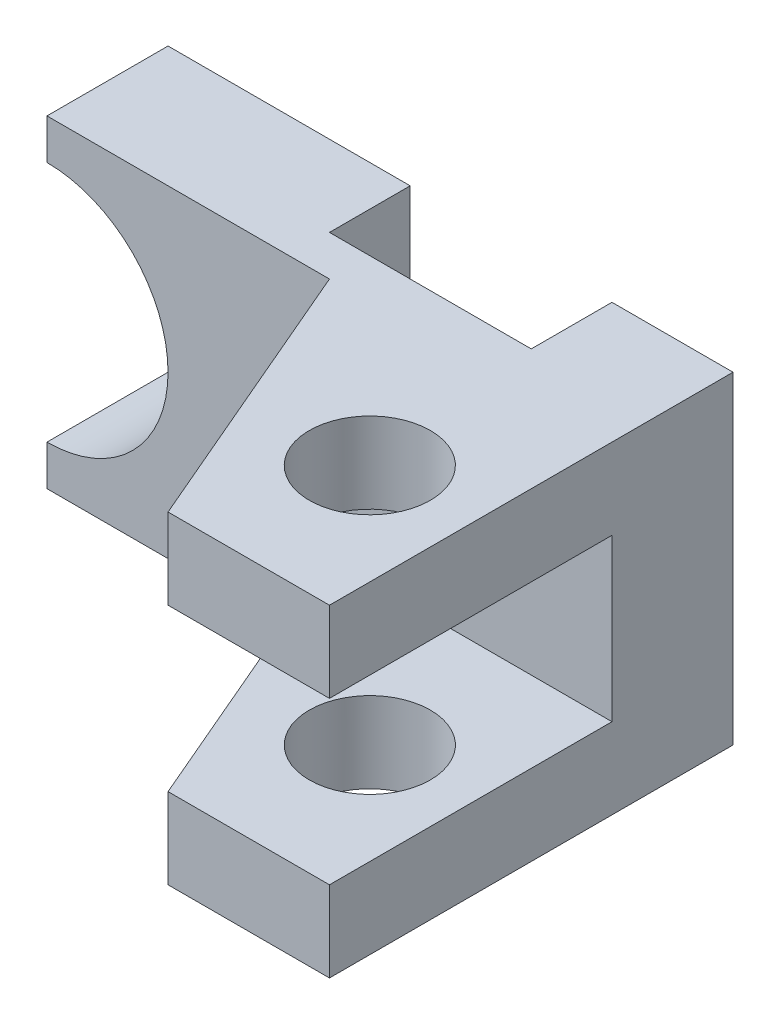
ISO-10303-21;
HEADER;
FILE_DESCRIPTION(('STEP AP214'),'2;1');
FILE_NAME('part.step','',(''),(''),'','','');
FILE_SCHEMA(('AUTOMOTIVE_DESIGN { 1 0 10303 214 1 1 1 1 }'));
ENDSEC;
DATA;
#1=APPLICATION_CONTEXT('core data for automotive mechanical design processes');
#2=APPLICATION_PROTOCOL_DEFINITION('international standard','automotive_design',2000,#1);
#3=PRODUCT_CONTEXT('',#1,'mechanical');
#4=PRODUCT('Part','Part','',(#3));
#5=PRODUCT_RELATED_PRODUCT_CATEGORY('part','',(#4));
#6=PRODUCT_DEFINITION_FORMATION('','',#4);
#7=PRODUCT_DEFINITION_CONTEXT('part definition',#1,'design');
#8=PRODUCT_DEFINITION('design','',#6,#7);
#9=PRODUCT_DEFINITION_SHAPE('','',#8);
#10=(LENGTH_UNIT() NAMED_UNIT(*) SI_UNIT(.MILLI.,.METRE.));
#11=(NAMED_UNIT(*) PLANE_ANGLE_UNIT() SI_UNIT($,.RADIAN.));
#12=(NAMED_UNIT(*) SI_UNIT($,.STERADIAN.) SOLID_ANGLE_UNIT());
#13=UNCERTAINTY_MEASURE_WITH_UNIT(LENGTH_MEASURE(1.E-05),#10,'distance_accuracy_value','');
#14=(GEOMETRIC_REPRESENTATION_CONTEXT(3) GLOBAL_UNCERTAINTY_ASSIGNED_CONTEXT((#13)) GLOBAL_UNIT_ASSIGNED_CONTEXT((#10,
#11,#12)) REPRESENTATION_CONTEXT('',''));
#15=CARTESIAN_POINT('',(0.,0.,0.));
#16=DIRECTION('',(0.,0.,1.));
#17=DIRECTION('',(1.,0.,0.));
#18=AXIS2_PLACEMENT_3D('',#15,#16,#17);
#19=CARTESIAN_POINT('',(0.,0.,0.));
#20=DIRECTION('',(0.,0.,1.));
#21=DIRECTION('',(1.,0.,0.));
#22=AXIS2_PLACEMENT_3D('',#19,#20,#21);
#23=PLANE('',#22);
#24=DIRECTION('',(-1.,0.,0.));
#25=VECTOR('',#24,1.);
#26=CARTESIAN_POINT('',(0.,0.,0.));
#27=LINE('',#26,#25);
#28=CARTESIAN_POINT('',(60.,0.,0.));
#29=VERTEX_POINT('',#28);
#30=CARTESIAN_POINT('',(0.,0.,0.));
#31=VERTEX_POINT('',#30);
#32=EDGE_CURVE('E279',#29,#31,#27,.T.);
#33=ORIENTED_EDGE('',*,*,#32,.F.);
#34=DIRECTION('',(0.,-1.,0.));
#35=VECTOR('',#34,1.);
#36=CARTESIAN_POINT('',(60.,0.,0.));
#37=LINE('',#36,#35);
#38=CARTESIAN_POINT('',(60.,-80.,0.));
#39=VERTEX_POINT('',#38);
#40=EDGE_CURVE('E192',#29,#39,#37,.T.);
#41=ORIENTED_EDGE('',*,*,#40,.T.);
#42=DIRECTION('',(1.,0.,0.));
#43=VECTOR('',#42,1.);
#44=CARTESIAN_POINT('',(0.,-80.,0.));
#45=LINE('',#44,#43);
#46=CARTESIAN_POINT('',(0.,-80.,0.));
#47=VERTEX_POINT('',#46);
#48=EDGE_CURVE('E272',#47,#39,#45,.T.);
#49=ORIENTED_EDGE('',*,*,#48,.F.);
#50=DIRECTION('',(0.,-1.,0.));
#51=VECTOR('',#50,1.);
#52=CARTESIAN_POINT('',(0.,0.,0.));
#53=LINE('',#52,#51);
#54=CARTESIAN_POINT('',(0.,-70.,0.));
#55=VERTEX_POINT('',#54);
#56=EDGE_CURVE('E269',#55,#47,#53,.T.);
#57=ORIENTED_EDGE('',*,*,#56,.F.);
#58=CARTESIAN_POINT('',(0.,-40.,0.));
#59=DIRECTION('',(0.,0.,1.));
#60=DIRECTION('',(1.,0.,0.));
#61=AXIS2_PLACEMENT_3D('',#58,#59,#60);
#62=CIRCLE('',#61,30.);
#63=CARTESIAN_POINT('',(0.,-10.,0.));
#64=VERTEX_POINT('',#63);
#65=EDGE_CURVE('E246',#55,#64,#62,.T.);
#66=ORIENTED_EDGE('',*,*,#65,.T.);
#67=EDGE_CURVE('E256',#31,#64,#53,.T.);
#68=ORIENTED_EDGE('',*,*,#67,.F.);
#69=EDGE_LOOP('',(#33,#41,#49,#57,#66,#68));
#70=FACE_BOUND('',#69,.T.);
#71=ADVANCED_FACE('F50',(#70),#23,.F.);
#72=CARTESIAN_POINT('',(0.,-40.,30.));
#73=DIRECTION('',(0.,0.,-1.));
#74=DIRECTION('',(-1.,0.,0.));
#75=AXIS2_PLACEMENT_3D('',#72,#73,#74);
#76=CYLINDRICAL_SURFACE('',#75,30.);
#77=ORIENTED_EDGE('',*,*,#65,.F.);
#78=DIRECTION('',(0.,0.,-1.));
#79=VECTOR('',#78,1.);
#80=CARTESIAN_POINT('',(0.,-70.,30.));
#81=LINE('',#80,#79);
#82=CARTESIAN_POINT('',(0.,-70.,30.));
#83=VERTEX_POINT('',#82);
#84=EDGE_CURVE('E11',#83,#55,#81,.T.);
#85=ORIENTED_EDGE('',*,*,#84,.F.);
#86=CARTESIAN_POINT('',(0.,-40.,30.));
#87=DIRECTION('',(0.,0.,1.));
#88=DIRECTION('',(1.,0.,0.));
#89=AXIS2_PLACEMENT_3D('',#86,#87,#88);
#90=CIRCLE('',#89,30.);
#91=CARTESIAN_POINT('',(0.,-10.,30.));
#92=VERTEX_POINT('',#91);
#93=EDGE_CURVE('E255',#83,#92,#90,.T.);
#94=ORIENTED_EDGE('',*,*,#93,.T.);
#95=DIRECTION('',(0.,0.,-1.));
#96=VECTOR('',#95,1.);
#97=CARTESIAN_POINT('',(0.,-10.,30.));
#98=LINE('',#97,#96);
#99=EDGE_CURVE('E278',#92,#64,#98,.T.);
#100=ORIENTED_EDGE('',*,*,#99,.T.);
#101=EDGE_LOOP('',(#77,#85,#94,#100));
#102=FACE_BOUND('',#101,.T.);
#103=ADVANCED_FACE('F47',(#102),#76,.F.);
#104=CARTESIAN_POINT('',(0.,0.,30.));
#105=DIRECTION('',(1.,0.,0.));
#106=DIRECTION('',(0.,0.,-1.));
#107=AXIS2_PLACEMENT_3D('',#104,#105,#106);
#108=PLANE('',#107);
#109=ORIENTED_EDGE('',*,*,#56,.T.);
#110=DIRECTION('',(0.,0.,-1.));
#111=VECTOR('',#110,1.);
#112=CARTESIAN_POINT('',(0.,-80.,30.));
#113=LINE('',#112,#111);
#114=CARTESIAN_POINT('',(0.,-80.,30.));
#115=VERTEX_POINT('',#114);
#116=EDGE_CURVE('E57',#115,#47,#113,.T.);
#117=ORIENTED_EDGE('',*,*,#116,.F.);
#118=DIRECTION('',(0.,-1.,0.));
#119=VECTOR('',#118,1.);
#120=CARTESIAN_POINT('',(0.,0.,30.));
#121=LINE('',#120,#119);
#122=EDGE_CURVE('E260',#83,#115,#121,.T.);
#123=ORIENTED_EDGE('',*,*,#122,.F.);
#124=ORIENTED_EDGE('',*,*,#84,.T.);
#125=EDGE_LOOP('',(#109,#117,#123,#124));
#126=FACE_BOUND('',#125,.T.);
#127=ADVANCED_FACE('F361',(#126),#108,.F.);
#128=CARTESIAN_POINT('',(0.,-80.,30.));
#129=DIRECTION('',(0.,1.,0.));
#130=DIRECTION('',(0.,0.,1.));
#131=AXIS2_PLACEMENT_3D('',#128,#129,#130);
#132=PLANE('',#131);
#133=CARTESIAN_POINT('',(115.,-80.,65.));
#134=DIRECTION('',(0.,-1.,0.));
#135=DIRECTION('',(0.,0.,-1.));
#136=AXIS2_PLACEMENT_3D('',#133,#134,#135);
#137=CIRCLE('',#136,15.);
#138=CARTESIAN_POINT('',(115.,-80.,50.));
#139=VERTEX_POINT('',#138);
#140=EDGE_CURVE('E191',#139,#139,#137,.T.);
#141=ORIENTED_EDGE('',*,*,#140,.F.);
#142=EDGE_LOOP('',(#141));
#143=FACE_BOUND('',#142,.T.);
#144=ORIENTED_EDGE('',*,*,#48,.T.);
#145=DIRECTION('',(0.,0.,-1.));
#146=VECTOR('',#145,1.);
#147=CARTESIAN_POINT('',(60.,-80.,20.));
#148=LINE('',#147,#146);
#149=CARTESIAN_POINT('',(60.,-80.,20.));
#150=VERTEX_POINT('',#149);
#151=EDGE_CURVE('E181',#150,#39,#148,.T.);
#152=ORIENTED_EDGE('',*,*,#151,.F.);
#153=DIRECTION('',(-1.,0.,0.));
#154=VECTOR('',#153,1.);
#155=CARTESIAN_POINT('',(110.,-80.,20.));
#156=LINE('',#155,#154);
#157=CARTESIAN_POINT('',(110.,-80.,20.));
#158=VERTEX_POINT('',#157);
#159=EDGE_CURVE('E183',#158,#150,#156,.T.);
#160=ORIENTED_EDGE('',*,*,#159,.F.);
#161=DIRECTION('',(0.,0.,1.));
#162=VECTOR('',#161,1.);
#163=CARTESIAN_POINT('',(110.,-80.,0.));
#164=LINE('',#163,#162);
#165=CARTESIAN_POINT('',(110.,-80.,0.));
#166=VERTEX_POINT('',#165);
#167=EDGE_CURVE('E162',#166,#158,#164,.T.);
#168=ORIENTED_EDGE('',*,*,#167,.F.);
#169=CARTESIAN_POINT('',(140.,-80.,0.));
#170=VERTEX_POINT('',#169);
#171=EDGE_CURVE('E275',#166,#170,#45,.T.);
#172=ORIENTED_EDGE('',*,*,#171,.T.);
#173=DIRECTION('',(0.,0.,-1.));
#174=VECTOR('',#173,1.);
#175=CARTESIAN_POINT('',(140.,-80.,30.));
#176=LINE('',#175,#174);
#177=CARTESIAN_POINT('',(140.,-80.,100.));
#178=VERTEX_POINT('',#177);
#179=EDGE_CURVE('E289',#178,#170,#176,.T.);
#180=ORIENTED_EDGE('',*,*,#179,.F.);
#181=DIRECTION('',(-1.,0.,0.));
#182=VECTOR('',#181,1.);
#183=CARTESIAN_POINT('',(140.,-80.,100.));
#184=LINE('',#183,#182);
#185=CARTESIAN_POINT('',(100.,-80.,100.));
#186=VERTEX_POINT('',#185);
#187=EDGE_CURVE('E223',#178,#186,#184,.T.);
#188=ORIENTED_EDGE('',*,*,#187,.T.);
#189=DIRECTION('',(-0.393919298579168,0.,-0.919145030018058));
#190=VECTOR('',#189,1.);
#191=CARTESIAN_POINT('',(70.,-80.,30.));
#192=LINE('',#191,#190);
#193=CARTESIAN_POINT('',(70.,-80.,30.));
#194=VERTEX_POINT('',#193);
#195=EDGE_CURVE('E235',#186,#194,#192,.T.);
#196=ORIENTED_EDGE('',*,*,#195,.T.);
#197=DIRECTION('',(1.,0.,0.));
#198=VECTOR('',#197,1.);
#199=CARTESIAN_POINT('',(0.,-80.,30.));
#200=LINE('',#199,#198);
#201=EDGE_CURVE('E257',#115,#194,#200,.T.);
#202=ORIENTED_EDGE('',*,*,#201,.F.);
#203=ORIENTED_EDGE('',*,*,#116,.T.);
#204=EDGE_LOOP('',(#144,#152,#160,#168,#172,#180,#188,#196,#202,#203));
#205=FACE_BOUND('',#204,.T.);
#206=ADVANCED_FACE('F293',(#143,#205),#132,.F.);
#207=CARTESIAN_POINT('',(140.,0.,30.));
#208=DIRECTION('',(-1.,0.,0.));
#209=DIRECTION('',(0.,0.,1.));
#210=AXIS2_PLACEMENT_3D('',#207,#208,#209);
#211=PLANE('',#210);
#212=DIRECTION('',(0.,1.,0.));
#213=VECTOR('',#212,1.);
#214=CARTESIAN_POINT('',(140.,0.,0.));
#215=LINE('',#214,#213);
#216=CARTESIAN_POINT('',(140.,0.,0.));
#217=VERTEX_POINT('',#216);
#218=EDGE_CURVE('E277',#170,#217,#215,.T.);
#219=ORIENTED_EDGE('',*,*,#218,.T.);
#220=DIRECTION('',(0.,0.,-1.));
#221=VECTOR('',#220,1.);
#222=CARTESIAN_POINT('',(140.,0.,30.));
#223=LINE('',#222,#221);
#224=CARTESIAN_POINT('',(140.,0.,100.));
#225=VERTEX_POINT('',#224);
#226=EDGE_CURVE('E282',#225,#217,#223,.T.);
#227=ORIENTED_EDGE('',*,*,#226,.F.);
#228=DIRECTION('',(0.,1.,0.));
#229=VECTOR('',#228,1.);
#230=CARTESIAN_POINT('',(140.,-20.,100.));
#231=LINE('',#230,#229);
#232=CARTESIAN_POINT('',(140.,-20.,100.));
#233=VERTEX_POINT('',#232);
#234=EDGE_CURVE('E225',#233,#225,#231,.T.);
#235=ORIENTED_EDGE('',*,*,#234,.F.);
#236=DIRECTION('',(0.,0.,-1.));
#237=VECTOR('',#236,1.);
#238=CARTESIAN_POINT('',(140.,-20.,30.));
#239=LINE('',#238,#237);
#240=CARTESIAN_POINT('',(140.,-20.,30.));
#241=VERTEX_POINT('',#240);
#242=EDGE_CURVE('E212',#233,#241,#239,.T.);
#243=ORIENTED_EDGE('',*,*,#242,.T.);
#244=DIRECTION('',(0.,1.,0.));
#245=VECTOR('',#244,1.);
#246=CARTESIAN_POINT('',(140.,0.,30.));
#247=LINE('',#246,#245);
#248=CARTESIAN_POINT('',(140.,-60.,30.));
#249=VERTEX_POINT('',#248);
#250=EDGE_CURVE('E262',#249,#241,#247,.T.);
#251=ORIENTED_EDGE('',*,*,#250,.F.);
#252=DIRECTION('',(0.,0.,1.));
#253=VECTOR('',#252,1.);
#254=CARTESIAN_POINT('',(140.,-60.,30.));
#255=LINE('',#254,#253);
#256=CARTESIAN_POINT('',(140.,-60.,100.));
#257=VERTEX_POINT('',#256);
#258=EDGE_CURVE('E234',#249,#257,#255,.T.);
#259=ORIENTED_EDGE('',*,*,#258,.T.);
#260=DIRECTION('',(0.,-1.,0.));
#261=VECTOR('',#260,1.);
#262=CARTESIAN_POINT('',(140.,-60.,100.));
#263=LINE('',#262,#261);
#264=EDGE_CURVE('E245',#257,#178,#263,.T.);
#265=ORIENTED_EDGE('',*,*,#264,.T.);
#266=ORIENTED_EDGE('',*,*,#179,.T.);
#267=EDGE_LOOP('',(#219,#227,#235,#243,#251,#259,#265,#266));
#268=FACE_BOUND('',#267,.T.);
#269=ADVANCED_FACE('F324',(#268),#211,.F.);
#270=CARTESIAN_POINT('',(0.,0.,30.));
#271=DIRECTION('',(0.,-1.,0.));
#272=DIRECTION('',(0.,0.,-1.));
#273=AXIS2_PLACEMENT_3D('',#270,#271,#272);
#274=PLANE('',#273);
#275=CARTESIAN_POINT('',(115.,0.,65.));
#276=DIRECTION('',(0.,-1.,0.));
#277=DIRECTION('',(0.,0.,-1.));
#278=AXIS2_PLACEMENT_3D('',#275,#276,#277);
#279=CIRCLE('',#278,15.);
#280=CARTESIAN_POINT('',(115.,0.,50.));
#281=VERTEX_POINT('',#280);
#282=EDGE_CURVE('E197',#281,#281,#279,.T.);
#283=ORIENTED_EDGE('',*,*,#282,.T.);
#284=EDGE_LOOP('',(#283));
#285=FACE_BOUND('',#284,.T.);
#286=DIRECTION('',(-1.,0.,0.));
#287=VECTOR('',#286,1.);
#288=CARTESIAN_POINT('',(110.,0.,20.));
#289=LINE('',#288,#287);
#290=CARTESIAN_POINT('',(110.,0.,20.));
#291=VERTEX_POINT('',#290);
#292=CARTESIAN_POINT('',(60.,0.,20.));
#293=VERTEX_POINT('',#292);
#294=EDGE_CURVE('E173',#291,#293,#289,.T.);
#295=ORIENTED_EDGE('',*,*,#294,.T.);
#296=DIRECTION('',(0.,0.,-1.));
#297=VECTOR('',#296,1.);
#298=CARTESIAN_POINT('',(60.,0.,20.));
#299=LINE('',#298,#297);
#300=EDGE_CURVE('E177',#293,#29,#299,.T.);
#301=ORIENTED_EDGE('',*,*,#300,.T.);
#302=ORIENTED_EDGE('',*,*,#32,.T.);
#303=DIRECTION('',(0.,0.,-1.));
#304=VECTOR('',#303,1.);
#305=CARTESIAN_POINT('',(0.,0.,30.));
#306=LINE('',#305,#304);
#307=CARTESIAN_POINT('',(0.,0.,30.));
#308=VERTEX_POINT('',#307);
#309=EDGE_CURVE('E285',#308,#31,#306,.T.);
#310=ORIENTED_EDGE('',*,*,#309,.F.);
#311=DIRECTION('',(-1.,0.,0.));
#312=VECTOR('',#311,1.);
#313=CARTESIAN_POINT('',(0.,0.,30.));
#314=LINE('',#313,#312);
#315=CARTESIAN_POINT('',(70.,0.,30.));
#316=VERTEX_POINT('',#315);
#317=EDGE_CURVE('E266',#316,#308,#314,.T.);
#318=ORIENTED_EDGE('',*,*,#317,.F.);
#319=DIRECTION('',(0.393919298579168,0.,0.919145030018058));
#320=VECTOR('',#319,1.);
#321=CARTESIAN_POINT('',(100.,0.,100.));
#322=LINE('',#321,#320);
#323=CARTESIAN_POINT('',(100.,0.,100.));
#324=VERTEX_POINT('',#323);
#325=EDGE_CURVE('E202',#316,#324,#322,.T.);
#326=ORIENTED_EDGE('',*,*,#325,.T.);
#327=DIRECTION('',(1.,0.,0.));
#328=VECTOR('',#327,1.);
#329=CARTESIAN_POINT('',(140.,0.,100.));
#330=LINE('',#329,#328);
#331=EDGE_CURVE('E208',#324,#225,#330,.T.);
#332=ORIENTED_EDGE('',*,*,#331,.T.);
#333=ORIENTED_EDGE('',*,*,#226,.T.);
#334=CARTESIAN_POINT('',(110.,0.,0.));
#335=VERTEX_POINT('',#334);
#336=EDGE_CURVE('E185',#217,#335,#27,.T.);
#337=ORIENTED_EDGE('',*,*,#336,.T.);
#338=DIRECTION('',(0.,0.,1.));
#339=VECTOR('',#338,1.);
#340=CARTESIAN_POINT('',(110.,0.,0.));
#341=LINE('',#340,#339);
#342=EDGE_CURVE('E61',#335,#291,#341,.T.);
#343=ORIENTED_EDGE('',*,*,#342,.T.);
#344=EDGE_LOOP('',(#295,#301,#302,#310,#318,#326,#332,#333,#337,#343));
#345=FACE_BOUND('',#344,.T.);
#346=ADVANCED_FACE('F176',(#285,#345),#274,.F.);
#347=ORIENTED_EDGE('',*,*,#67,.T.);
#348=ORIENTED_EDGE('',*,*,#99,.F.);
#349=EDGE_CURVE('E261',#308,#92,#121,.T.);
#350=ORIENTED_EDGE('',*,*,#349,.F.);
#351=ORIENTED_EDGE('',*,*,#309,.T.);
#352=EDGE_LOOP('',(#347,#348,#350,#351));
#353=FACE_BOUND('',#352,.T.);
#354=ADVANCED_FACE('F309',(#353),#108,.F.);
#355=CARTESIAN_POINT('',(0.,0.,30.));
#356=DIRECTION('',(0.,0.,1.));
#357=DIRECTION('',(1.,0.,0.));
#358=AXIS2_PLACEMENT_3D('',#355,#356,#357);
#359=PLANE('',#358);
#360=DIRECTION('',(0.,1.,0.));
#361=VECTOR('',#360,1.);
#362=CARTESIAN_POINT('',(70.,-20.,30.));
#363=LINE('',#362,#361);
#364=CARTESIAN_POINT('',(70.,-20.,30.));
#365=VERTEX_POINT('',#364);
#366=EDGE_CURVE('E220',#365,#316,#363,.T.);
#367=ORIENTED_EDGE('',*,*,#366,.T.);
#368=ORIENTED_EDGE('',*,*,#317,.T.);
#369=ORIENTED_EDGE('',*,*,#349,.T.);
#370=ORIENTED_EDGE('',*,*,#93,.F.);
#371=ORIENTED_EDGE('',*,*,#122,.T.);
#372=ORIENTED_EDGE('',*,*,#201,.T.);
#373=DIRECTION('',(0.,-1.,0.));
#374=VECTOR('',#373,1.);
#375=CARTESIAN_POINT('',(70.,-60.,30.));
#376=LINE('',#375,#374);
#377=CARTESIAN_POINT('',(70.,-60.,30.));
#378=VERTEX_POINT('',#377);
#379=EDGE_CURVE('E249',#378,#194,#376,.T.);
#380=ORIENTED_EDGE('',*,*,#379,.F.);
#381=DIRECTION('',(1.,0.,0.));
#382=VECTOR('',#381,1.);
#383=CARTESIAN_POINT('',(140.,-60.,30.));
#384=LINE('',#383,#382);
#385=EDGE_CURVE('E229',#378,#249,#384,.T.);
#386=ORIENTED_EDGE('',*,*,#385,.T.);
#387=ORIENTED_EDGE('',*,*,#250,.T.);
#388=DIRECTION('',(-1.,0.,0.));
#389=VECTOR('',#388,1.);
#390=CARTESIAN_POINT('',(70.,-20.,30.));
#391=LINE('',#390,#389);
#392=EDGE_CURVE('E72',#241,#365,#391,.T.);
#393=ORIENTED_EDGE('',*,*,#392,.T.);
#394=EDGE_LOOP('',(#367,#368,#369,#370,#371,#372,#380,#386,#387,#393));
#395=FACE_BOUND('',#394,.T.);
#396=ADVANCED_FACE('F314',(#395),#359,.T.);
#397=ORIENTED_EDGE('',*,*,#171,.F.);
#398=DIRECTION('',(0.,-1.,0.));
#399=VECTOR('',#398,1.);
#400=CARTESIAN_POINT('',(110.,0.,0.));
#401=LINE('',#400,#399);
#402=EDGE_CURVE('E169',#335,#166,#401,.T.);
#403=ORIENTED_EDGE('',*,*,#402,.F.);
#404=ORIENTED_EDGE('',*,*,#336,.F.);
#405=ORIENTED_EDGE('',*,*,#218,.F.);
#406=EDGE_LOOP('',(#397,#403,#404,#405));
#407=FACE_BOUND('',#406,.T.);
#408=ADVANCED_FACE('F329',(#407),#23,.F.);
#409=CARTESIAN_POINT('',(70.,-60.,30.));
#410=DIRECTION('',(-0.919145030018058,0.,0.393919298579168));
#411=DIRECTION('',(0.393919298579168,0.,0.919145030018058));
#412=AXIS2_PLACEMENT_3D('',#409,#410,#411);
#413=PLANE('',#412);
#414=ORIENTED_EDGE('',*,*,#195,.F.);
#415=DIRECTION('',(0.,-1.,0.));
#416=VECTOR('',#415,1.);
#417=CARTESIAN_POINT('',(100.,-60.,100.));
#418=LINE('',#417,#416);
#419=CARTESIAN_POINT('',(100.,-60.,100.));
#420=VERTEX_POINT('',#419);
#421=EDGE_CURVE('E248',#420,#186,#418,.T.);
#422=ORIENTED_EDGE('',*,*,#421,.F.);
#423=DIRECTION('',(-0.393919298579168,0.,-0.919145030018058));
#424=VECTOR('',#423,1.);
#425=CARTESIAN_POINT('',(70.,-60.,30.));
#426=LINE('',#425,#424);
#427=EDGE_CURVE('E239',#420,#378,#426,.T.);
#428=ORIENTED_EDGE('',*,*,#427,.T.);
#429=ORIENTED_EDGE('',*,*,#379,.T.);
#430=EDGE_LOOP('',(#414,#422,#428,#429));
#431=FACE_BOUND('',#430,.T.);
#432=ADVANCED_FACE('F340',(#431),#413,.T.);
#433=CARTESIAN_POINT('',(140.,-60.,100.));
#434=DIRECTION('',(0.,0.,1.));
#435=DIRECTION('',(1.,0.,0.));
#436=AXIS2_PLACEMENT_3D('',#433,#434,#435);
#437=PLANE('',#436);
#438=ORIENTED_EDGE('',*,*,#187,.F.);
#439=ORIENTED_EDGE('',*,*,#264,.F.);
#440=DIRECTION('',(-1.,0.,0.));
#441=VECTOR('',#440,1.);
#442=CARTESIAN_POINT('',(140.,-60.,100.));
#443=LINE('',#442,#441);
#444=EDGE_CURVE('E237',#257,#420,#443,.T.);
#445=ORIENTED_EDGE('',*,*,#444,.T.);
#446=ORIENTED_EDGE('',*,*,#421,.T.);
#447=EDGE_LOOP('',(#438,#439,#445,#446));
#448=FACE_BOUND('',#447,.T.);
#449=ADVANCED_FACE('F331',(#448),#437,.T.);
#450=CARTESIAN_POINT('',(0.,-60.,0.));
#451=DIRECTION('',(0.,1.,0.));
#452=DIRECTION('',(0.,0.,1.));
#453=AXIS2_PLACEMENT_3D('',#450,#451,#452);
#454=PLANE('',#453);
#455=CARTESIAN_POINT('',(115.,-60.,65.));
#456=DIRECTION('',(0.,1.,0.));
#457=DIRECTION('',(0.,0.,1.));
#458=AXIS2_PLACEMENT_3D('',#455,#456,#457);
#459=CIRCLE('',#458,15.);
#460=CARTESIAN_POINT('',(115.,-60.,80.));
#461=VERTEX_POINT('',#460);
#462=EDGE_CURVE('E205',#461,#461,#459,.T.);
#463=ORIENTED_EDGE('',*,*,#462,.F.);
#464=EDGE_LOOP('',(#463));
#465=FACE_BOUND('',#464,.T.);
#466=ORIENTED_EDGE('',*,*,#385,.F.);
#467=ORIENTED_EDGE('',*,*,#427,.F.);
#468=ORIENTED_EDGE('',*,*,#444,.F.);
#469=ORIENTED_EDGE('',*,*,#258,.F.);
#470=EDGE_LOOP('',(#466,#467,#468,#469));
#471=FACE_BOUND('',#470,.T.);
#472=ADVANCED_FACE('F342',(#465,#471),#454,.T.);
#473=CARTESIAN_POINT('',(140.,-20.,100.));
#474=DIRECTION('',(0.,0.,1.));
#475=DIRECTION('',(1.,0.,0.));
#476=AXIS2_PLACEMENT_3D('',#473,#474,#475);
#477=PLANE('',#476);
#478=ORIENTED_EDGE('',*,*,#331,.F.);
#479=DIRECTION('',(0.,1.,0.));
#480=VECTOR('',#479,1.);
#481=CARTESIAN_POINT('',(100.,-20.,100.));
#482=LINE('',#481,#480);
#483=CARTESIAN_POINT('',(100.,-20.,100.));
#484=VERTEX_POINT('',#483);
#485=EDGE_CURVE('E228',#484,#324,#482,.T.);
#486=ORIENTED_EDGE('',*,*,#485,.F.);
#487=DIRECTION('',(1.,0.,0.));
#488=VECTOR('',#487,1.);
#489=CARTESIAN_POINT('',(140.,-20.,100.));
#490=LINE('',#489,#488);
#491=EDGE_CURVE('E211',#484,#233,#490,.T.);
#492=ORIENTED_EDGE('',*,*,#491,.T.);
#493=ORIENTED_EDGE('',*,*,#234,.T.);
#494=EDGE_LOOP('',(#478,#486,#492,#493));
#495=FACE_BOUND('',#494,.T.);
#496=ADVANCED_FACE('F325',(#495),#477,.T.);
#497=CARTESIAN_POINT('',(100.,-20.,100.));
#498=DIRECTION('',(-0.919145030018058,0.,0.393919298579168));
#499=DIRECTION('',(0.393919298579168,0.,0.919145030018058));
#500=AXIS2_PLACEMENT_3D('',#497,#498,#499);
#501=PLANE('',#500);
#502=ORIENTED_EDGE('',*,*,#325,.F.);
#503=ORIENTED_EDGE('',*,*,#366,.F.);
#504=DIRECTION('',(0.393919298579168,0.,0.919145030018058));
#505=VECTOR('',#504,1.);
#506=CARTESIAN_POINT('',(100.,-20.,100.));
#507=LINE('',#506,#505);
#508=EDGE_CURVE('E210',#365,#484,#507,.T.);
#509=ORIENTED_EDGE('',*,*,#508,.T.);
#510=ORIENTED_EDGE('',*,*,#485,.T.);
#511=EDGE_LOOP('',(#502,#503,#509,#510));
#512=FACE_BOUND('',#511,.T.);
#513=ADVANCED_FACE('F318',(#512),#501,.T.);
#514=CARTESIAN_POINT('',(0.,-20.,0.));
#515=DIRECTION('',(0.,-1.,0.));
#516=DIRECTION('',(0.,0.,-1.));
#517=AXIS2_PLACEMENT_3D('',#514,#515,#516);
#518=PLANE('',#517);
#519=CARTESIAN_POINT('',(115.,-20.,65.));
#520=DIRECTION('',(0.,-1.,0.));
#521=DIRECTION('',(0.,0.,-1.));
#522=AXIS2_PLACEMENT_3D('',#519,#520,#521);
#523=CIRCLE('',#522,15.);
#524=CARTESIAN_POINT('',(115.,-20.,50.));
#525=VERTEX_POINT('',#524);
#526=EDGE_CURVE('E51',#525,#525,#523,.T.);
#527=ORIENTED_EDGE('',*,*,#526,.F.);
#528=EDGE_LOOP('',(#527));
#529=FACE_BOUND('',#528,.T.);
#530=ORIENTED_EDGE('',*,*,#392,.F.);
#531=ORIENTED_EDGE('',*,*,#242,.F.);
#532=ORIENTED_EDGE('',*,*,#491,.F.);
#533=ORIENTED_EDGE('',*,*,#508,.F.);
#534=EDGE_LOOP('',(#530,#531,#532,#533));
#535=FACE_BOUND('',#534,.T.);
#536=ADVANCED_FACE('F401',(#529,#535),#518,.T.);
#537=CARTESIAN_POINT('',(115.,0.,65.));
#538=DIRECTION('',(0.,-1.,0.));
#539=DIRECTION('',(0.,0.,-1.));
#540=AXIS2_PLACEMENT_3D('',#537,#538,#539);
#541=CYLINDRICAL_SURFACE('',#540,15.);
#542=ORIENTED_EDGE('',*,*,#526,.T.);
#543=EDGE_LOOP('',(#542));
#544=FACE_BOUND('',#543,.T.);
#545=ORIENTED_EDGE('',*,*,#282,.F.);
#546=EDGE_LOOP('',(#545));
#547=FACE_BOUND('',#546,.T.);
#548=ADVANCED_FACE('F397',(#544,#547),#541,.F.);
#549=ORIENTED_EDGE('',*,*,#462,.T.);
#550=EDGE_LOOP('',(#549));
#551=FACE_BOUND('',#550,.T.);
#552=ORIENTED_EDGE('',*,*,#140,.T.);
#553=EDGE_LOOP('',(#552));
#554=FACE_BOUND('',#553,.T.);
#555=ADVANCED_FACE('F394',(#551,#554),#541,.F.);
#556=CARTESIAN_POINT('',(60.,0.,20.));
#557=DIRECTION('',(-1.,0.,0.));
#558=DIRECTION('',(0.,0.,1.));
#559=AXIS2_PLACEMENT_3D('',#556,#557,#558);
#560=PLANE('',#559);
#561=ORIENTED_EDGE('',*,*,#151,.T.);
#562=ORIENTED_EDGE('',*,*,#40,.F.);
#563=ORIENTED_EDGE('',*,*,#300,.F.);
#564=DIRECTION('',(0.,-1.,0.));
#565=VECTOR('',#564,1.);
#566=CARTESIAN_POINT('',(60.,0.,20.));
#567=LINE('',#566,#565);
#568=EDGE_CURVE('E170',#293,#150,#567,.T.);
#569=ORIENTED_EDGE('',*,*,#568,.T.);
#570=EDGE_LOOP('',(#561,#562,#563,#569));
#571=FACE_BOUND('',#570,.T.);
#572=ADVANCED_FACE('F303',(#571),#560,.F.);
#573=CARTESIAN_POINT('',(110.,0.,20.));
#574=DIRECTION('',(0.,0.,1.));
#575=DIRECTION('',(1.,0.,0.));
#576=AXIS2_PLACEMENT_3D('',#573,#574,#575);
#577=PLANE('',#576);
#578=ORIENTED_EDGE('',*,*,#159,.T.);
#579=ORIENTED_EDGE('',*,*,#568,.F.);
#580=ORIENTED_EDGE('',*,*,#294,.F.);
#581=DIRECTION('',(0.,-1.,0.));
#582=VECTOR('',#581,1.);
#583=CARTESIAN_POINT('',(110.,0.,20.));
#584=LINE('',#583,#582);
#585=EDGE_CURVE('E157',#291,#158,#584,.T.);
#586=ORIENTED_EDGE('',*,*,#585,.T.);
#587=EDGE_LOOP('',(#578,#579,#580,#586));
#588=FACE_BOUND('',#587,.T.);
#589=ADVANCED_FACE('F175',(#588),#577,.F.);
#590=CARTESIAN_POINT('',(110.,0.,0.));
#591=DIRECTION('',(1.,0.,0.));
#592=DIRECTION('',(0.,0.,-1.));
#593=AXIS2_PLACEMENT_3D('',#590,#591,#592);
#594=PLANE('',#593);
#595=ORIENTED_EDGE('',*,*,#167,.T.);
#596=ORIENTED_EDGE('',*,*,#585,.F.);
#597=ORIENTED_EDGE('',*,*,#342,.F.);
#598=ORIENTED_EDGE('',*,*,#402,.T.);
#599=EDGE_LOOP('',(#595,#596,#597,#598));
#600=FACE_BOUND('',#599,.T.);
#601=ADVANCED_FACE('F161',(#600),#594,.F.);
#602=CLOSED_SHELL('',(#71,#103,#127,#206,#269,#346,#354,#396,#408,#432,#449,#472,#496,#513,#536,
#548,#555,#572,#589,#601));
#603=MANIFOLD_SOLID_BREP('B2',#602);
#604=ADVANCED_BREP_SHAPE_REPRESENTATION('',(#18,#603),#14);
#605=SHAPE_DEFINITION_REPRESENTATION(#9,#604);
ENDSEC;
END-ISO-10303-21;
